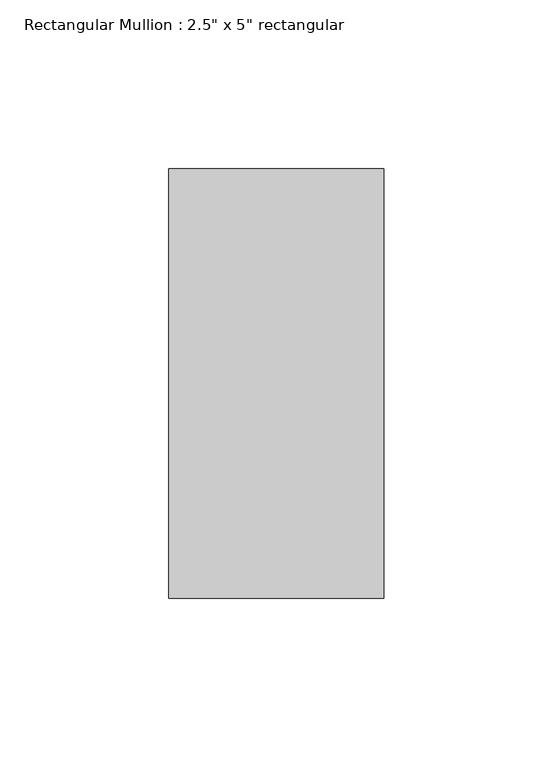
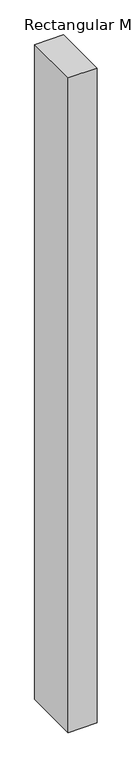
"""IFC4 building model written with IfcOpenShell, lengths in millimetres: member geometry."""

from ifc_helpers import new_model, si_unit, frame, origin, place, context, project, spatial, polyline, outline, extrude, source, transform, mapped, element, save


def member_44b7b902(model_context):
    return source(origin(), model_context, "Body", "SweptSolid", [
        extrude(outline(polyline([(0.0, 63.5), (0.0, -63.5), (-63.5, -63.5), (-63.5, 63.5), (0.0, 63.5)])), frame((0.0, 0.0, -1516.4056705), z_axis=(0.0, 0.0, 1.0), x_axis=(1.0, 0.0, 0.0)), (0.0, 0.0, 1.0), 1516.4056705),
    ])


if __name__ == "__main__":
    model = new_model("IFC4")
    model_context = context("Model", 3, world=origin())
    ifc_project = project(units=[si_unit("LENGTHUNIT", "METRE", prefix="MILLI")], contexts=[model_context])
    site = spatial("IfcSite", under=ifc_project)
    building = spatial("IfcBuilding", under=site)
    placement = place(None, origin())
    member_shape = member_44b7b902(model_context)
    element("IfcMember", 1, ObjectType="Rectangular Mullion : 2.5\" x 5\" rectangular", at=placement, inside=building, context=model_context, shape_type="MappedRepresentation", body=[
        mapped(member_shape, transform((0.0, 0.0, 0.0), x_axis=(1.0, 0.0, 0.0), y_axis=(0.0, 1.0, 0.0), z_axis=(0.0, 0.0, 1.0))),
    ])
    save(model, "model.ifc")

# Revit data of these elements
# Type "Rectangular Mullion : 2.5\" x 5\" rectangular"
#   built-in parameter 1007304 = 0.416667 (stored number, unit not read)
#   built-in parameter 1007301 = 0.104167 (stored number, unit not read)
#   built-in parameter 1007300 = 0.104167 (stored number, unit not read)
# Element 1 (IfcMember, "Rectangular Mullion : 2.5\" x 5\" rectangular")
#   Materials on its faces: "Aluminum"
# Materials
#   "Aluminum": class "Metal", colour RGB 247 247 247, transparency 0, Description = "Aluminum 6061", Cost = 0
